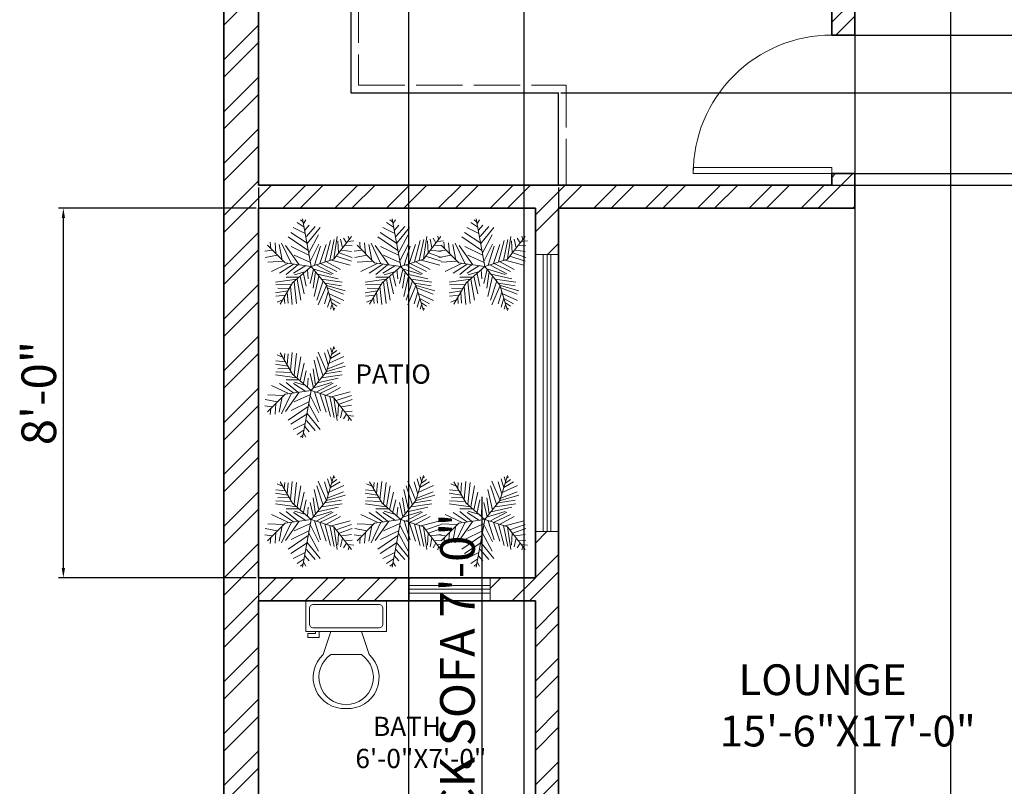
# Model space of a CAD drawing. Units: inches. Extents: x 177 to 1423, y 532 to 2503.
# Tile 2 of 5: x 197 to 453, y 897 to 1096. Entities that reach past the tile are written whole.
import ezdxf

# ---------------------------------------------------------------- set-up
doc = ezdxf.new("R2010")
doc.units = ezdxf.units.IN
doc.linetypes.add('ACAD_ISO02W100', pattern=[15, 12, -3])
for name, color, linetype, lineweight in [('A-ANNO-DIMS', 2, 'Continuous', 18), ('A-AREA-IDEN', 7, 'Continuous', 18), ('A-DOOR', 4, 'Continuous', 18), ('A-FLOR-CASE', 8, 'Continuous', 25), ('A-FLOR-CASE-HIDN', 8, 'ACAD_ISO02W100', 13), ('A-FLOR-FIXT', 9, 'Continuous', 18), ('A-GLAZ', 244, 'Continuous', 18), ('A-WALL', 7, 'Continuous', 35), ('A-WALL-PATT', 252, 'Continuous', 13), ('L-PLNT', 94, 'Continuous', 13)]:
    doc.layers.add(name, color=color, linetype=linetype, lineweight=lineweight)
doc.styles.get("Standard").update_dxf_attribs({"font": 'arial.ttf'})
doc.dimstyles.new('ISO-25', dxfattribs={"dimtxt": 9, "dimasz": 2.5, "dimexe": 1.25, "dimexo": 0.625, "dimtad": 1, "dimlunit": 3, "dimtxsty": 'Standard', "dimcen": 2.5, "dimadec": 0, "dimazin": 0, "dimtfac": 1, "dimtmove": 0, "dimatfit": 3, "dimfxl": 1, "dimarcsym": 0})

# ---------------------------------------------------------------- blocks, each defined once
blk = doc.blocks.new('*U6')
for p, q in [((0, 0), (0, 6)), ((40, 0), (40, 6))]:
    blk.add_line(p, q)
blk.add_lwpolyline([(0, 0), (0, -40), (1.75, -40), (1.75, 0)], close=True)
blk.add_arc((0, 0), 40, 270, 0)
blk = doc.blocks.new('*U9')
for p, q in [((9.5, -6), (9.5, -2)), ((-10, -8.5), (-8, -8.5)), ((-10, -9.5), (-10, -8.5)), ((-7, -9.5), (-10, -9.5)), ((-8, -8.5), (-8, -8)), ((-7, -8), (-7, -9.5)), ((-4, -8), (-6, -14)), ((4, -8), (6, -14)), ((4, -14), (-4, -14))]:
    blk.add_line(p, q)
blk.add_lwpolyline([(10.5, -8), (10.5, 0), (-10.5, 0), (-10.5, -8)], close=True)
for points in [[(-9.5, -2), (-9.5, -6)], [(8.5, -1), (-8.5, -1)], [(-8.5, -7), (8.5, -7)]]:
    blk.add_lwpolyline(points)
for centre, radius, start, end in [((-8.625, -1.875), 0.8839, 81.8699, 188.1301), ((8.625, -1.875), 0.8839, 351.8699, 98.1301), ((-8.625, -6.125), 0.8839, 171.869898, 278.1301), ((8.625, -6.125), 0.8839, 261.8699, 8.1301), ((-0.4772, -19.9188), 8.0953, 133.01722, 273.38), ((0.0374, -19.8731), 7.127, 124.50543, 269.7), ((-0.0373, -19.8731), 7.127, 270.3, 55.4946), ((0.4773, -19.9188), 8.0953, 266.62, 46.9828)]:
    blk.add_arc(centre, radius, start, end)
blk = doc.blocks.new('*U11')
for p, q in [((-8.737, 47.138), (-17.069, 52.711)), ((-10.186, 53.64), (-13.084, 55.962)), ((0, 0), (-10.5, 57)), ((-9.099, 51.782), (-6.563, 55.962)), ((-7.65, 43.423), (-2.578, 49.46)), ((-5.839, 35.992), (4.667, 48.067)), ((-3.665, 19.273), (-27.574, 35.527)), ((-5.114, 28.097), (-24.676, 40.636)), ((-7.288, 39.707), (-21.778, 46.673)), ((-5.114, 27.632), (10.463, 46.673)), ((-2.941, 16.486), (8.652, 37.85)), ((27, 9), (48, 36)), ((27.127, 9.056), (31.112, 35.992)), ((44.153, 36.456), (45.239, 32.741)), ((-31.5, 4.5), (-52.5, 25.5)), ((-48.585, 21.131), (-49.309, 29.026)), ((-43.513, 28.561), (-42.427, 15.558)), ((-38.442, 26.239), (-34.819, 7.663)), ((-35.544, 28.097), (-24.314, 3.947)), ((-14.533, 2.09), (-30.834, 25.31)), ((-24.314, 23.917), (-2.941, 13.7)), ((-1.129, 6.734), (9.014, 26.704)), ((3.942, 1.625), (11.187, 24.381)), ((10.101, 3.483), (17.708, 26.239)), ((16.259, 5.805), (23.142, 31.348)), ((22.055, 7.198), (27.489, 32.277)), ((31.836, 30.883), (32.561, 16.486)), ((35.096, 32.741), (37.27, 22.524)), ((38.719, 34.134), (41.979, 28.561)), ((40.53, 25.775), (48.862, 24.846)), ((43.791, 29.954), (51.036, 30.883)), ((-47.498, 19.737), (-55.83, 18.344)), ((-40.615, 13.7), (-55.105, 10.913)), ((-20.691, 13.7), (-1.129, 4.876)), ((29.662, 12.307), (48.137, 6.269)), ((33.285, 16.486), (48.862, 10.913)), ((36.183, 19.737), (48.137, 17.88)), ((-33.37, 6.269), (-52.207, 5.34)), ((-28.299, 3.483), (-47.86, -5.805)), ((-21.416, 3.018), (-38.079, -8.128)), ((0, 0), (-31.5, 4.5)), ((-15.982, 2.09), (-30.11, -9.521)), ((0, 0), (-22.5, -19.5)), ((-6.563, 1.161), (-21.416, -8.128)), ((0, 0), (27, 9)), ((0, 0), (18, -22.5)), ((6.478, 1.625), (26.04, -8.592)), ((11.187, 3.483), (30.749, -5.805)), ((18.07, 5.805), (35.096, -3.483)), ((24.229, 7.663), (46.688, 1.625)), ((-6.563, -5.805), (-19.967, -9.985)), ((-13.446, -11.378), (-8.737, -32.741)), ((-9.461, -8.592), (-6.201, -23.453)), ((-4.752, -3.483), (-3.665, -14.629)), ((2.493, -3.019), (-1.491, -20.202)), ((1.769, -2.555), (24.229, -9.521)), ((5.029, -6.27), (2.131, -25.775)), ((9.014, -11.378), (3.58, -35.992)), ((7.565, -9.056), (32.198, -14.629)), ((-17.431, -15.094), (-42.789, -18.809)), ((-24.314, -21.596), (-42.427, -22.06)), ((-22.5, -19.5), (-37.5, -45)), ((-15.257, -12.772), (-30.11, -12.772)), ((-20.691, -18.345), (-17.793, -44.352)), ((-17.069, -15.094), (-12.721, -40.172)), ((14.085, -16.951), (6.478, -40.172)), ((18.07, -22.524), (8.289, -45.745)), ((12.274, -15.094), (36.907, -18.809)), ((16.259, -19.738), (36.183, -22.989)), ((18, -22.5), (27, -52.5)), ((18.433, -22.524), (40.53, -29.026)), ((-28.299, -29.026), (-42.789, -31.348)), ((-30.834, -34.135), (-42.427, -35.528)), ((-26.849, -26.24), (-40.253, -25.775)), ((-29.023, -30.884), (-27.936, -43.887)), ((-25.038, -23.918), (-22.865, -45.281)), ((20.244, -30.419), (15.897, -44.816)), ((19.157, -25.311), (38.719, -33.206)), ((21.331, -32.741), (39.081, -40.636)), ((-34.457, -39.708), (-40.978, -42.494)), ((-32.646, -36.921), (-31.921, -44.352)), ((22.78, -37.85), (19.519, -48.532)), ((22.78, -38.314), (34.372, -44.816)), ((24.591, -45.745), (23.142, -50.854)), ((24.591, -43.423), (30.749, -47.603)), ((26.764, -49.925), (28.213, -50.854))]:
    blk.add_line(p, q)
blk = doc.blocks.new('WIN-GLAZING-72IN')
for p, q in [((72, 2), (0, 2)), ((72, 1), (0, 1)), ((72, 0), (0, 0))]:
    blk.add_line(p, q)
blk = doc.blocks.new('*D32')
at = {"layer": 'A-ANNO-DIMS', "color": 0, "lineweight": -2, "transparency": 16777216}
for p, q in [((317.7, 823.42), (317.7, 972.18)), ((305.73, 823.42), (318.95, 823.42)), ((317.7, 741.92), (317.7, 820.92)), ((305.73, 739.42), (318.95, 739.42))]:
    blk.add_line(p, q, dxfattribs=at)
at = {"layer": 'A-ANNO-DIMS', "color": 0, "transparency": 16777216}
for points in [[(317.29, 820.92), (318.12, 820.92), (317.7, 823.42)], [(317.29, 741.92), (318.12, 741.92), (317.7, 739.42)]]:
    blk.add_solid(points, dxfattribs=at)
at = {"layer": 'Defpoints', "color": 0, "transparency": 16777216}
for p in [(305.1, 823.42), (317.7, 823.42), (305.1, 739.42)]:
    blk.add_point(p, dxfattribs=at)
at = {"layer": 'A-ANNO-DIMS', "color": 0, "transparency": 16777216, "insert": (312.42, 899.05), "char_height": 9, "attachment_point": 5, "rotation": 90}
blk.add_mtext('ROUNDBACK SOFA 7\'-0"', dxfattribs=at)
blk = doc.blocks.new('*D39')
at = {"layer": 'A-ANNO-DIMS', "color": 0, "lineweight": -2, "transparency": 16777216}
for p, q in [((258.93, 1047.15), (207.55, 1047.15)), ((208.8, 953.65), (208.8, 1044.65)), ((258.93, 951.15), (207.55, 951.15))]:
    blk.add_line(p, q, dxfattribs=at)
at = {"layer": 'A-ANNO-DIMS', "color": 0, "transparency": 16777216}
for points in [[(208.38, 1044.65), (209.22, 1044.65), (208.8, 1047.15)], [(208.38, 953.65), (209.22, 953.65), (208.8, 951.15)]]:
    blk.add_solid(points, dxfattribs=at)
at = {"layer": 'Defpoints', "color": 0, "transparency": 16777216}
for p in [(208.8, 1047.15), (259.55, 1047.15), (259.55, 951.15)]:
    blk.add_point(p, dxfattribs=at)
at = {"layer": 'A-ANNO-DIMS', "color": 0, "transparency": 16777216, "insert": (203.58, 999.15), "char_height": 9, "attachment_point": 5, "rotation": 90}
blk.add_mtext('8\'-0"', dxfattribs=at)
blk = doc.blocks.new('*D40')
at = {"layer": 'A-ANNO-DIMS', "color": 0, "lineweight": -2, "transparency": 16777216}
for p, q in [((414.55, 1172.53), (414.55, 538.84)), ((505.55, 1172.53), (505.55, 538.84)), ((417.05, 540.09), (503.05, 540.09))]:
    blk.add_line(p, q, dxfattribs=at)
at = {"layer": 'A-ANNO-DIMS', "color": 0, "transparency": 16777216}
for points in [[(417.05, 540.51), (417.05, 539.68), (414.55, 540.09)], [(503.05, 540.51), (503.05, 539.68), (505.55, 540.09)]]:
    blk.add_solid(points, dxfattribs=at)
at = {"layer": 'Defpoints', "color": 0, "transparency": 16777216}
for p in [(414.55, 1173.15), (505.55, 1173.15), (505.55, 540.09)]:
    blk.add_point(p, dxfattribs=at)
at = {"layer": 'A-ANNO-DIMS', "color": 0, "transparency": 16777216, "insert": (460.05, 545.22), "char_height": 9, "attachment_point": 5}
blk.add_mtext('7\'-7"', dxfattribs=at)
blk = doc.blocks.new('*D41')
at = {"layer": 'A-ANNO-DIMS', "color": 0, "lineweight": -2, "transparency": 16777216}
for p, q in [((439.55, 861.78), (439.55, 1447.15)), ((499.55, 861.78), (499.55, 1447.15)), ((442.05, 1445.9), (497.05, 1445.9))]:
    blk.add_line(p, q, dxfattribs=at)
at = {"layer": 'A-ANNO-DIMS', "color": 0, "transparency": 16777216}
for points in [[(442.05, 1446.32), (442.05, 1445.49), (439.55, 1445.9)], [(497.05, 1446.32), (497.05, 1445.49), (499.55, 1445.9)]]:
    blk.add_solid(points, dxfattribs=at)
at = {"layer": 'Defpoints', "color": 0, "transparency": 16777216}
for p in [(499.55, 1445.9), (439.55, 861.15), (499.55, 861.15)]:
    blk.add_point(p, dxfattribs=at)
at = {"layer": 'A-ANNO-DIMS', "color": 0, "transparency": 16777216, "insert": (469.55, 1451.12), "char_height": 9, "attachment_point": 5}
blk.add_mtext('5\'-0"', dxfattribs=at)
blk = doc.blocks.new('*D48')
at = {"layer": 'A-ANNO-DIMS', "color": 0, "lineweight": -2, "transparency": 16777216}
for p, q in [((766.3, 1077.15), (766.3, 1104.98)), ((338.12, 1077.15), (767.55, 1077.15)), ((766.3, 1055.65), (766.3, 1074.65)), ((338.12, 1053.15), (767.55, 1053.15))]:
    blk.add_line(p, q, dxfattribs=at)
at = {"layer": 'A-ANNO-DIMS', "color": 0, "transparency": 16777216}
for points in [[(765.88, 1074.65), (766.72, 1074.65), (766.3, 1077.15)], [(765.88, 1055.65), (766.72, 1055.65), (766.3, 1053.15)]]:
    blk.add_solid(points, dxfattribs=at)
at = {"layer": 'Defpoints', "color": 0, "transparency": 16777216}
for p in [(337.49, 1077.15), (766.3, 1077.15), (337.49, 1053.15)]:
    blk.add_point(p, dxfattribs=at)
at = {"layer": 'A-ANNO-DIMS', "color": 0, "transparency": 16777216, "insert": (761.08, 1092.32), "char_height": 9, "attachment_point": 5, "rotation": 90}
blk.add_mtext('2\'-0"', dxfattribs=at)
blk = doc.blocks.new('*D49')
at = {"layer": 'A-ANNO-DIMS', "color": 0, "lineweight": -2, "transparency": 16777216}
for p, q in [((259.55, 1052.53), (259.55, 538.84)), ((337.49, 1052.53), (337.49, 538.84)), ((262.05, 540.09), (334.99, 540.09))]:
    blk.add_line(p, q, dxfattribs=at)
at = {"layer": 'A-ANNO-DIMS', "color": 0, "transparency": 16777216}
for points in [[(262.05, 540.51), (262.05, 539.68), (259.55, 540.09)], [(334.99, 540.51), (334.99, 539.68), (337.49, 540.09)]]:
    blk.add_solid(points, dxfattribs=at)
at = {"layer": 'Defpoints', "color": 0, "transparency": 16777216}
for p in [(259.55, 1053.15), (337.49, 1053.15), (337.49, 540.09)]:
    blk.add_point(p, dxfattribs=at)
at = {"layer": 'A-ANNO-DIMS', "color": 0, "transparency": 16777216, "insert": (298.52, 545.31), "char_height": 9, "attachment_point": 5}
blk.add_mtext('6\'-6"', dxfattribs=at)
blk = doc.blocks.new('*D52')
at = {"layer": 'A-ANNO-DIMS', "color": 0, "lineweight": -2, "transparency": 16777216}
for p, q in [((409.18, 1092.15), (767.55, 1092.15)), ((766.3, 1058.65), (766.3, 1089.65)), ((409.18, 1056.15), (767.55, 1056.15))]:
    blk.add_line(p, q, dxfattribs=at)
at = {"layer": 'A-ANNO-DIMS', "color": 0, "transparency": 16777216}
for points in [[(765.88, 1089.65), (766.72, 1089.65), (766.3, 1092.15)], [(765.88, 1058.65), (766.72, 1058.65), (766.3, 1056.15)]]:
    blk.add_solid(points, dxfattribs=at)
at = {"layer": 'Defpoints', "color": 0, "transparency": 16777216}
for p in [(408.55, 1092.15), (766.3, 1092.15), (408.55, 1056.15)]:
    blk.add_point(p, dxfattribs=at)
at = {"layer": 'A-ANNO-DIMS', "color": 0, "transparency": 16777216, "insert": (761.08, 1074.15), "char_height": 9, "attachment_point": 5, "rotation": 90}
blk.add_mtext('3\'-0"', dxfattribs=at)
blk = doc.blocks.new('*D56')
at = {"layer": 'A-ANNO-DIMS', "color": 0, "lineweight": -2, "transparency": 16777216}
for p, q in [((298.55, 1259.53), (298.55, 538.84)), ((328.55, 1259.53), (328.55, 538.84)), ((301.05, 540.09), (326.05, 540.09))]:
    blk.add_line(p, q, dxfattribs=at)
at = {"layer": 'A-ANNO-DIMS', "color": 0, "transparency": 16777216}
for points in [[(301.05, 540.51), (301.05, 539.68), (298.55, 540.09)], [(326.05, 540.51), (326.05, 539.68), (328.55, 540.09)]]:
    blk.add_solid(points, dxfattribs=at)
at = {"layer": 'Defpoints', "color": 0, "transparency": 16777216}
for p in [(298.55, 1260.15), (328.55, 1260.15), (328.55, 540.09)]:
    blk.add_point(p, dxfattribs=at)
at = {"layer": 'A-ANNO-DIMS', "color": 0, "transparency": 16777216, "insert": (313.55, 545.31), "char_height": 9, "attachment_point": 5}
blk.add_mtext('2\'-6"', dxfattribs=at)

msp = doc.modelspace()

# ---------------------------------------------------------------- hatches: boundary and pattern name
at = {"layer": 'A-WALL-PATT'}
h = msp.add_hatch(dxfattribs=at)
h.set_pattern_fill('ANSI32', color=256)
h.paths.add_polyline_path([(436.55, 810.154), (427.55, 810.154), (427.55, 711.154), (379.55, 711.154), (379.55, 702.154), (436.55, 702.154)])
h.paths.add_polyline_path([(337.55, 963.154), (331.55, 963.154), (331.55, 951.154), (319.738, 951.154), (319.738, 945.154), (331.55, 945.154), (331.55, 861.154), (328.55, 861.154), (328.55, 855.154), (427.55, 855.154), (427.55, 846.154), (436.55, 846.154), (436.55, 852.154), (439.55, 852.154), (439.55, 861.154), (337.55, 861.154)], flags=17)
h.paths.add_polyline_path([(682.55, 1011.154), (643.55, 1011.154), (643.55, 1095.154), (701.063, 1095.154), (701.063, 1101.154), (700.55, 1101.154), (700.55, 1143.154), (691.55, 1143.154), (691.55, 1101.154), (511.55, 1101.154), (511.55, 1104.154), (505.55, 1104.154), (505.55, 1068.154), (511.55, 1068.154), (511.55, 1095.154), (637.55, 1095.154), (637.55, 1011.154), (511.55, 1011.154), (511.55, 1038.154), (505.55, 1038.154), (505.55, 1005.154), (541.55, 1005.154), (541.55, 1002.154), (547.55, 1002.154), (547.55, 1005.154), (682.55, 1005.154)], flags=17)
h.paths.add_polyline_path([(547.55, 966.154), (541.55, 966.154), (541.55, 861.154), (499.55, 861.154), (499.55, 852.154), (595.55, 852.154), (595.55, 861.154), (547.55, 861.154)], flags=17)
h.paths.add_polyline_path([(724.55, 1353.154), (337.55, 1353.154), (250.55, 1353.154), (250.55, 702.154), (307.55, 702.154), (307.55, 711.154), (259.55, 711.154), (259.55, 855.154), (298.55, 855.154), (298.55, 861.154), (259.55, 861.154), (259.55, 945.154), (298.738, 945.154), (298.738, 951.154), (259.55, 951.154), (259.55, 1047.154), (331.55, 1047.154), (331.55, 1035.154), (337.55, 1035.154), (337.55, 1047.154), (414.55, 1047.154), (414.55, 1056.154), (408.55, 1056.154), (408.55, 1053.154), (259.55, 1053.154), (259.55, 1173.154), (408.55, 1173.154), (408.55, 1092.154), (414.55, 1092.154), (414.55, 1173.154), (466.55, 1173.154), (466.55, 1179.154), (337.55, 1179.154), (337.55, 1194.154), (331.55, 1194.154), (331.55, 1179.154), (259.55, 1179.154), (259.55, 1194.154), (259.55, 1254.154), (298.55, 1254.154), (298.55, 1258.654), (298.55, 1260.154), (259.55, 1260.154), (259.55, 1344.154), (331.55, 1344.154), (331.55, 1346.691), (337.55, 1346.691), (337.55, 1347.154), (637.55, 1347.154), (637.55, 1346.676), (643.55, 1346.676), (643.55, 1344.154), (715.55, 1344.154), (715.55, 1263.154), (643.55, 1263.154), (643.55, 1266.154), (642.05, 1266.154), (637.55, 1266.154), (637.55, 1263.154), (610.55, 1263.154), (610.55, 1257.154), (691.55, 1257.154), (691.55, 1215.154), (700.55, 1215.154), (700.55, 1257.154), (718.55, 1257.154), (718.55, 1101.154), (715.137, 1101.154), (715.137, 1095.154), (715.55, 1095.154), (715.55, 1011.154), (712.55, 1011.154), (712.55, 1009.654), (712.55, 1005.154), (715.55, 1005.154), (715.55, 861.154), (667.55, 861.154), (667.55, 852.154), (724.55, 852.154)])
h.paths.add_polyline_path([(571.243, 1332.154), (457.55, 1332.154), (457.55, 1323.154), (505.55, 1323.154), (505.55, 1179.154), (502.55, 1179.154), (502.55, 1178.554), (502.55, 1173.154), (505.55, 1173.154), (505.55, 1140.154), (510.95, 1140.154), (511.55, 1140.154), (511.55, 1257.154), (574.55, 1257.154), (574.55, 1263.154), (511.55, 1263.154), (511.55, 1323.154), (571.243, 1323.154)], flags=17)
h.paths.add_polyline_path([(385.55, 1332.154), (337.55, 1332.154), (337.55, 1332.617), (331.55, 1332.617), (331.55, 1260.154), (328.55, 1260.154), (328.55, 1254.154), (337.55, 1254.154), (337.55, 1323.154), (385.55, 1323.154)], flags=17)
h.paths.add_polyline_path([(643.55, 1332.601), (637.55, 1332.601), (637.55, 1332.154), (607.243, 1332.154), (607.243, 1323.154), (637.55, 1323.154), (637.55, 1296.154), (642.05, 1296.154), (643.55, 1296.154)], flags=17)

# ---------------------------------------------------------------- linework, layer by layer
at = {"layer": 'A-DOOR'}
msp.add_line((414.55, 1092.154), (414.55, 1056.154), dxfattribs=at)
at = {"layer": 'A-FLOR-CASE'}
for p, q in [((283.55, 1149.154), (283.55, 1077.154)), ((283.55, 1077.154), (337.493, 1077.154)), ((337.493, 1053.154), (337.493, 1077.154))]:
    msp.add_line(p, q, dxfattribs=at)
at = {"layer": 'A-FLOR-CASE-HIDN'}
for p, q in [((285.55, 1147.154), (285.55, 1079.154)), ((285.55, 1079.154), (339.493, 1079.154)), ((339.493, 1053.154), (339.493, 1079.154))]:
    msp.add_line(p, q, dxfattribs=at)
at = {"layer": 'A-GLAZ'}
for p, q in [((298.738, 949.154), (319.738, 949.154)), ((298.738, 948.154), (319.738, 948.154)), ((298.738, 947.154), (319.738, 947.154))]:
    msp.add_line(p, q, dxfattribs=at)
for points in [[(337.55, 1035.154), (337.55, 963.154), (331.55, 963.154), (331.55, 1035.154)], [(298.738, 951.154), (319.738, 951.154), (319.738, 945.154), (298.738, 945.154)]]:
    msp.add_lwpolyline(points, close=True, dxfattribs=at)
at = {"layer": 'A-WALL'}
for p, q in [((250.55, 1353.154), (250.55, 636.154)), ((259.55, 1173.154), (259.55, 1053.154)), ((408.55, 1173.154), (408.55, 1092.154)), ((414.55, 1173.154), (414.55, 1092.154)), ((408.55, 1092.154), (414.55, 1092.154)), ((408.55, 1056.154), (414.55, 1056.154)), ((408.55, 1056.154), (408.55, 1053.154)), ((414.55, 1056.154), (414.55, 1047.154)), ((259.55, 1053.154), (408.55, 1053.154)), ((259.55, 1047.154), (331.55, 1047.154)), ((259.55, 1047.154), (259.55, 951.154)), ((331.55, 1047.154), (331.55, 951.154)), ((337.55, 1047.154), (337.55, 861.154)), ((337.55, 1047.154), (414.55, 1047.154)), ((259.55, 951.154), (331.55, 951.154)), ((259.55, 945.154), (331.55, 945.154)), ((259.55, 945.154), (259.55, 861.154)), ((331.55, 945.154), (331.55, 861.154))]:
    msp.add_line(p, q, dxfattribs=at)

# ---------------------------------------------------------------- block references
at = {"layer": 'A-DOOR', "xscale": -0.9000000000000095, "yscale": 0.9000000000000095, "zscale": 0.9000000000000095, "rotation": 270}
msp.add_blockref('*U6', (408.55, 1056.154), dxfattribs=at)
at = {"layer": 'A-FLOR-FIXT'}
msp.add_blockref('*U9', (282.323, 945.154), dxfattribs=at)
at = {"layer": 'A-GLAZ', "rotation": 270.0000000000013}
msp.add_blockref('WIN-GLAZING-72IN', (333.55, 1035.155), dxfattribs=at)
at = {"layer": 'L-PLNT', "xscale": 0.2170156140567048, "yscale": 0.2170156140567048, "zscale": 0.2170156140567048}
for p in [(273.268, 1032.011), (296.548, 1032.011), (318.413, 1032.011)]:
    msp.add_blockref('*U11', p, dxfattribs=at)
at = {"layer": 'L-PLNT', "xscale": -0.2170156140567048, "yscale": 0.2170156140567048, "zscale": 0.2170156140567048, "rotation": 180}
for p in [(273.268, 999.828), (273.268, 966.297), (296.548, 966.297), (318.413, 966.297)]:
    msp.add_blockref('*U11', p, dxfattribs=at)

# ---------------------------------------------------------------- texts
at = {"layer": 'A-AREA-IDEN', "attachment_point": 1}
for s, width, insert, char_height in [('PATIO', 22.74319, (284.72, 1006.566), 5), ('  LOUNGE\\P15\'-6"X17\'-0"', 64.26677, (379.42, 928.632), 8), ('   BATH\\P6\'-0"X7\'-0"', 34.04512, (284.72, 915.01), 5)]:
    msp.add_mtext_dynamic_manual_height_columns(s, width=width, gutter_width=12.5, heights=[0], dxfattribs=dict(at, insert=insert, char_height=char_height))

# ---------------------------------------------------------------- dimensions: what is measured, and where the dimension line sits
at = {"layer": 'A-ANNO-DIMS'}
for base, p1, p2, picture, middle in [((499.55, 1445.904), (439.55, 861.154), (499.55, 861.154), '*D41', (469.55, 1451.124)), ((328.55, 540.092), (298.55, 1260.154), (328.55, 1260.154), '*D56', (313.55, 545.313)), ((505.55, 540.092), (414.55, 1173.154), (505.55, 1173.154), '*D40', (460.05, 545.217)), ((337.493, 540.092), (259.55, 1053.154), (337.493, 1053.154), '*D49', (298.522, 545.313))]:
    dim = msp.add_linear_dim(base=base, p1=p1, p2=p2, dimstyle='ISO-25', override={"dimdec": 1, "dimlfac": 1, "dimrnd": 0, "dimzin": 1, "dimdsep": 46, "dimlunit": 4, "dimfrac": 2}, dxfattribs=at)
    dim.commit()
    dim.dimension.update_dxf_attribs({"geometry": picture, "text_midpoint": middle})
for base, p1, p2, picture, middle in [((766.3, 1077.154), (337.493, 1053.154), (337.493, 1077.154), '*D48', (761.08, 1092.318)), ((766.3, 1092.154), (408.55, 1056.154), (408.55, 1092.154), '*D52', (761.077, 1074.154)), ((208.8, 1047.154), (259.55, 951.154), (259.55, 1047.154), '*D39', (203.58, 999.154))]:
    dim = msp.add_linear_dim(base=base, p1=p1, p2=p2, angle=90, dimstyle='ISO-25', override={"dimdec": 1, "dimlfac": 1, "dimrnd": 0, "dimzin": 1, "dimdsep": 46, "dimlunit": 4, "dimfrac": 2}, dxfattribs=at)
    dim.commit()
    dim.dimension.update_dxf_attribs({"geometry": picture, "text_midpoint": middle})
dim = msp.add_linear_dim(base=(317.703, 823.419), p1=(305.103, 739.419), p2=(305.103, 823.419), angle=90, text='ROUNDBACK SOFA <>', dimstyle='ISO-25', override={"dimdec": 1, "dimlfac": 1, "dimrnd": 0, "dimzin": 1, "dimdsep": 46, "dimlunit": 4, "dimfrac": 2}, dxfattribs=at)
dim.commit()
dim.dimension.update_dxf_attribs({"geometry": '*D32', "text_midpoint": (312.422, 899.051)})

doc.saveas('drawing.dxf')
